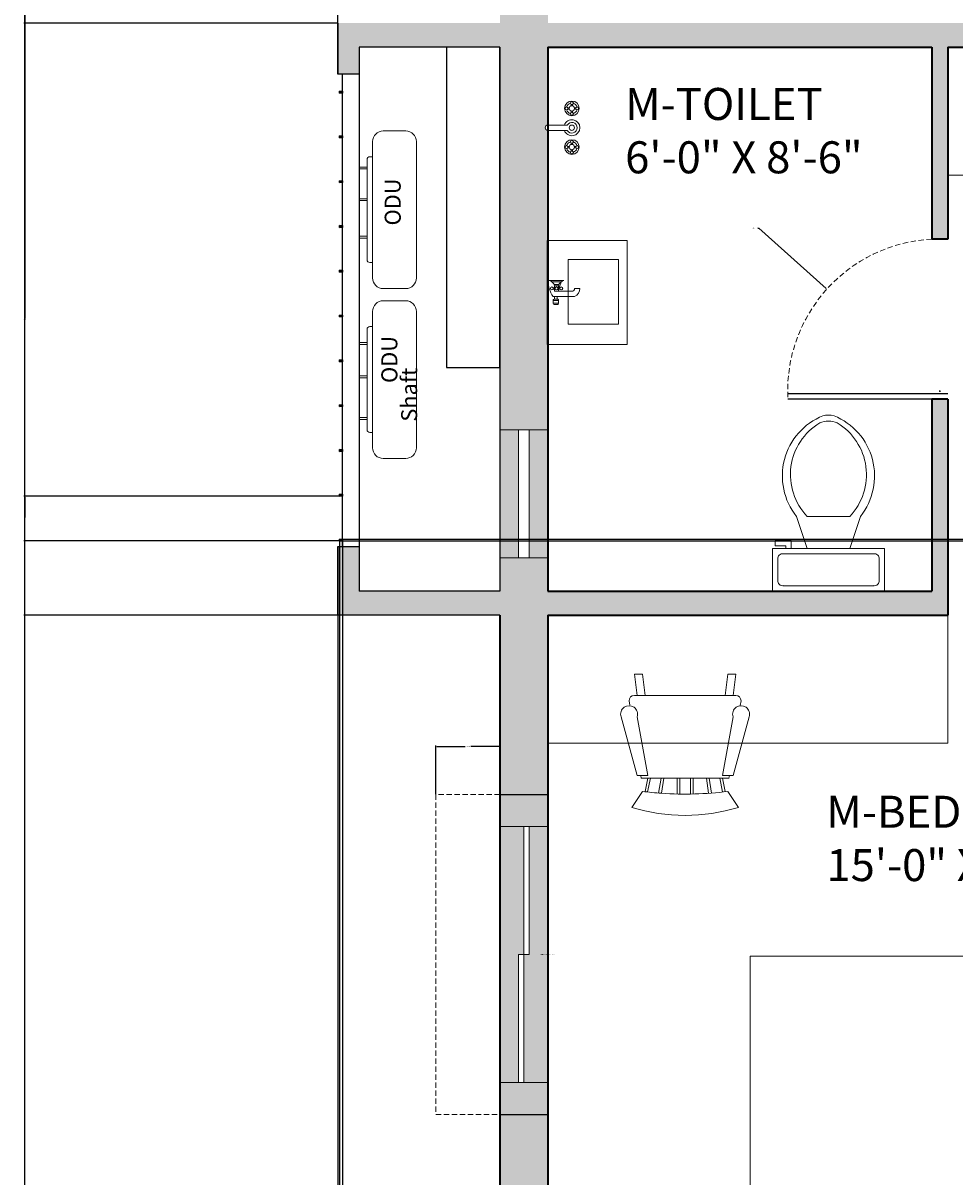
# Model space of a CAD drawing. Units: inches. Extents: x 1693 to 2974, y 2201 to 2965.
# Tile 2 of 24: x 1693 to 1868, y 2337 to 2554. Entities that reach past the tile are written whole.
import ezdxf

# ---------------------------------------------------------------- set-up
doc = ezdxf.new("R2010")
doc.units = ezdxf.units.IN
doc.header["$LTSCALE"] = 2
doc.header["$MEASUREMENT"] = 0
doc.linetypes.add('HIDDEN', pattern=[0.375, 0.25, -0.125])
for name, color, linetype, lineweight in [('A-ANNO-DIMS', 2, 'Continuous', 18), ('A-ANNO-TEXT', 7, 'Continuous', 13), ('A-AREA-IDEN', 7, 'Continuous', 18), ('A-DOOR', 3, 'Continuous', 25), ('A-DOOR-SWNG', 3, 'HIDDEN', 13), ('A-FLOR-CASE', 32, 'Continuous', 18), ('A-FLOR-FIXT', 9, 'Continuous', 18), ('A-FLOR-SHFT', 7, 'Continuous', 25), ('A-FURN', 8, 'Continuous', 18), ('A-GLAZ', 4, 'Continuous', 18), ('A-GLAZ-OVHD', 8, 'HIDDEN', 13), ('A-WALL', 7, 'Continuous', 35), ('M-HVAC-EQPM', 151, 'Continuous', 18)]:
    doc.layers.add(name, color=color, linetype=linetype, lineweight=lineweight)
doc.layers.add('A-GLAZ-PATT', color=141, linetype='Continuous', lineweight=13, true_color=0xadddf7)
doc.layers.add('A-WALL-PATT', color=251, linetype='Continuous', lineweight=13, true_color=0x636466)
doc.styles.get("Standard").update_dxf_attribs({"font": 'arial.ttf'})
doc.dimstyles.get("Standard").update_dxf_attribs({"dimtxt": 0.18, "dimasz": 0.18, "dimexe": 0.18, "dimexo": 0.0625, "dimgap": 0.09, "dimtad": 0, "dimtih": 1, "dimtoh": 1, "dimdec": 1, "dimzin": 0, "dimdsep": 46, "dimlunit": 3, "dimtxsty": 'Standard', "dimcen": 0.09, "dimadec": 0, "dimazin": 0, "dimtfac": 1, "dimtdec": 1, "dimtofl": 0, "dimtmove": 0, "dimatfit": 3, "dimfxl": 1, "dimtolj": 1, "dimtzin": 0, "dimarcsym": 0})

# ---------------------------------------------------------------- blocks, each defined once
blk = doc.blocks.new('Bed - Queen')
for p, q in [((0, -80.00003), (0, 0)), ((0, 0), (59.99999, 0)), ((59.99999, 0), (59.99999, -80.00003)), ((7.99999, -1.2), (28.79998, -1.2)), ((7.99999, -14.4), (7.99999, -1.2)), ((28.79998, -1.2), (28.79998, -14.4)), ((31.19999, -1.2), (51.99999, -1.2)), ((31.19999, -14.4), (31.19999, -1.2)), ((51.99999, -1.2), (51.99999, -16.4)), ((0, -14.4), (44.8, -14.4)), ((59.99999, -29.6), (44.8, -14.4)), ((44.8, -14.4), (44.8, -29.6)), ((44.8, -16.8), (0, -16.8)), ((51.99999, -16.4), (46.79936, -16.4)), ((44.8, -29.6), (59.99999, -29.6)), ((59.99999, -80.00003), (0, -80.00003))]:
    blk.add_line(p, q)
blk = doc.blocks.new('Toilet - top')
for p, q in [((9.5, -6), (9.5, -2)), ((-10, -8.5), (-8, -8.5)), ((-10, -9.5), (-10, -8.5)), ((-8, -8.5), (-8, -8)), ((-7, -8), (-7, -9.5)), ((-4, -8), (-6, -14)), ((4, -8), (6, -14)), ((-7, -9.5), (-10, -9.5)), ((4, -14), (-4, -14))]:
    blk.add_line(p, q)
blk.add_lwpolyline([(10.5, -8), (10.5, 0), (-10.5, 0), (-10.5, -8)], close=True)
for points in [[(-9.5, -2), (-9.5, -6)], [(8.5, -1), (-8.5, -1)], [(-8.5, -7), (8.5, -7)]]:
    blk.add_lwpolyline(points)
for centre, radius, start, end in [((-8.62, -1.88), 0.884, 81.8699, 188.1301), ((8.62, -1.88), 0.884, 351.8699, 98.1301), ((-8.62, -6.12), 0.884, 171.8699, 278.1301), ((8.62, -6.12), 0.884, 261.8699, 8.1301), ((3.52, -21.58), 12.17, 141.4691, 247.9714), ((4.2, -21.82), 11.33, 136.3677, 238.9468), ((-3.52, -21.58), 12.17, 292.0284, 38.5307), ((-4.2, -21.82), 11.33, 301.053, 43.6321), ((0, -27.88), 4, 245.7318, 294.2682), ((0, -29), 4, 254.8605, 285.1395)]:
    blk.add_arc(centre, radius, start, end)
blk = doc.blocks.new('Faucet - Bathroom side')
for p, q in [((-0.625, 4.25), (0.375, 4.25)), ((0.375, 3.75), (-0.625, 3.75)), ((-0.625, 3), (3.375, 3)), ((-0.375, 3), (-0.375, 3.5)), ((0.125, 3.5), (0.125, 3)), ((-1.625, 0), (-1.375, 0)), ((-1.375, 0), (1.375, 0)), ((-0.88366, 0.25), (0.88424, 0.25)), ((-0.375, 1.625), (-0.625, 1.625)), ((-0.375, 1.375), (-0.625, 1.375)), ((0.48078, 0.75), (-0.47286, 0.75)), ((2.875, 2), (0.375, 2)), ((0.375, 1.625), (0.625, 1.625)), ((0.375, 1.375), (0.625, 1.375)), ((4.375, 1.5), (3.375, 1.5))]:
    blk.add_line(p, q)
for points in [[(-0.375, 4.5), (0.125, 4.5)], [(-0.625, 3.75), (-0.625, 4.25)], [(0.125, 3.5), (-0.375, 3.5)], [(0.375, 4.25), (0.375, 3.75)]]:
    blk.add_lwpolyline(points)
blk.add_lwpolyline([(-0.375, 1), (-0.375, 2), (0.375, 2), (0.375, 1)], close=True)
for centre in [(-0.875, 1.5), (0, 1.5), (0.875, 1.5)]:
    blk.add_circle(centre, 0.27951)
for centre, radius, start, end in [((-0.38253, 4.2575), 0.24259, 88.22243, 181.7776), ((0.13252, 4.2575), 0.24259, 358.2224, 91.77757), ((3.45929, -0.0281), 5.08436, 143.4467, 179.6834), ((-0.38253, 3.7424), 0.24259, 178.2224, 271.7776), ((0.13252, 3.7424), 0.24259, 268.2224, 1.777565), ((2.70708, 1.4714), 1.66816, 0.9827695, 66.39737), ((-1.75, 1.375), 1.42522, 285.2551, 344.7449), ((1.75, 1.375), 1.42522, 195.2551, 254.7449), ((-2.49562, -0.286), 3.38273, 9.709485, 29.48735), ((2.96867, 1.5936), 0.41699, 347.0192, 102.9808)]:
    blk.add_arc(centre, radius, start, end)
blk = doc.blocks.new('Faucet - Bathroom top')
for p, q in [((-4.107, 0.125), (-4.375, 0.125)), ((-3.75, 0.4788), (-3.75, 0.75)), ((-3.5, 0.482), (-3.5, 0.75)), ((-3.1461, 0.125), (-2.875, 0.125)), ((3.143, 0.125), (2.875, 0.125)), ((3.5, 0.4788), (3.5, 0.75)), ((3.75, 0.482), (3.75, 0.75)), ((4.1039, 0.125), (4.375, 0.125)), ((-4.1039, -0.125), (-4.375, -0.125)), ((-3.75, -0.4821), (-3.75, -0.75)), ((-3.5, -0.4789), (-3.5, -0.75)), ((-3.143, -0.125), (-2.875, -0.125)), ((-0.5, -0.8639), (-0.5, -4.5)), ((0.5, -4.5), (0.5, -0.8631)), ((3.1461, -0.125), (2.875, -0.125)), ((3.5, -0.4821), (3.5, -0.75)), ((3.75, -0.4789), (3.75, -0.75)), ((4.107, -0.125), (4.375, -0.125))]:
    blk.add_line(p, q)
for centre, radius in [((-3.625, 0), 1.375), ((-4.625, 0), 0.2795), ((-3.625, 0), 0.5), ((-3.625, 1), 0.2795), ((-2.625, 0), 0.2795), ((0, 0), 0.5), ((3.625, 0), 1.375), ((2.625, 0), 0.2795), ((3.625, 0), 0.5), ((3.625, 1), 0.2795), ((4.625, 0), 0.2795), ((-3.625, -1), 0.2795), ((3.625, -1), 0.2795)]:
    blk.add_circle(centre, radius)
for centre, radius, start, end in [((-3.625, 0), 1, 105.2407, 164.2093), ((-3.625, 0), 1, 16.44125, 74.07887), ((0, 0), 1.5, 289.6514, 250.3603), ((0, 0), 1, 300.3431, 239.7554), ((3.625, 0), 1, 106.12, 164.0884), ((3.625, 0), 1, 16.23422, 73.90469), ((-3.625, 0), 1, 196.2342, 253.9047), ((-3.625, 0), 1, 286.12, 344.0884), ((3.625, 0), 1, 196.4413, 254.0789), ((3.625, 0), 1, 285.2407, 344.2093), ((0, -4.5), 0.5, 180, 0)]:
    blk.add_arc(centre, radius, start, end)
blk = doc.blocks.new('Chair - Rocking')
for p, q in [((-8, -4.5), (-10, -1.5)), ((8, -4.5), (10, -1.5)), ((-4.5, -7), (-4.96674, -4.19951)), ((-4, -7), (-4.40532, -4.16272)), ((-1.5, -4.05012), (-1.5, -7)), ((-1, -7), (-1, -4.05012)), ((1, -7), (1, -4.04655)), ((1.5, -4.05012), (1.5, -7)), ((4, -7), (4.40187, -4.18694)), ((4.5, -7), (4.96761, -4.19437)), ((-7.5, -4.5), (-7, -7)), ((-6.5, -7), (-7.02225, -4.43)), ((6.5, -7), (7, -4.4057)), ((7.5, -4.5), (7, -7)), ((-9, -7.5), (-12, -18.49999)), ((-7, -7.5), (-9, -7.5)), ((-9, -18.49999), (-7, -7.5)), ((-8.23428, -6.99939), (-8.3093, -7.47958)), ((-8.23041, -7), (8.23915, -7)), ((7, -7.5), (9, -7.5)), ((9, -18.49999), (7, -7.5)), ((8.31071, -7.48854), (8.23449, -7.00073)), ((9, -7.5), (12, -18.49999)), ((-10.36644, -20.64523), (-10.5, -21.49999)), ((10.5, -21.49999), (10.3575, -20.58798)), ((-9, -22.49999), (-9.5, -26.49999)), ((0, -22.49999), (-9.5, -22.49999)), ((-8, -26.49999), (-7.5, -22.49999)), ((0, -22.49999), (9.5, -22.49999)), ((8, -26.49999), (7.5, -22.49999)), ((9, -22.49999), (9.5, -26.49999)), ((-9.5, -26.49999), (-8, -26.49999)), ((9.5, -26.49999), (8, -26.49999))]:
    blk.add_line(p, q)
for centre, radius, start, end in [((0, -34.08333), 34.08333, 72.93847, 107.0615), ((0, -68.25004), 64.25, 93.92211, 97.15267), ((0, -68.25004), 64.25, 82.84733, 93.92211), ((-10.5, -18.99999), 1.58114, 161.5651, 18.43495), ((10.5, -18.99999), 1.58114, 161.5651, 18.43495), ((-9.5, -21.49999), 1, 180, 270), ((9.5, -21.49999), 1, 270, 0)]:
    blk.add_arc(centre, radius, start, end)
blk = doc.blocks.new('CONDENSER-WITH-BRACKETS')
at = {"ltscale": 2}
for points in [[(2, 10.74), (27.57, 10.74, -0.414214), (29.57, 8.74), (29.57, 4.53, -0.414214), (27.57, 2.53), (2, 2.53, -0.414214), (0, 4.53), (0, 8.74, -0.414214)], [(4.85, 2.53), (24.67, 2.53), (24.67, 2, -0.414214), (24.17, 1.5), (5.35, 1.5, -0.414214), (4.85, 2)]]:
    blk.add_lwpolyline(points, format="xyb", close=True, dxfattribs=at)
for points in [[(7.84, 1.5), (8.19, 1.5), (8.19, 0), (7.84, 0)], [(14.1, 1.5), (14.45, 1.5), (14.45, 0), (14.1, 0)], [(21.89, 1.5), (22.24, 1.5), (22.24, 0), (21.89, 0)]]:
    blk.add_lwpolyline(points, close=True, dxfattribs=at)
blk = doc.blocks.new('SHAFT-GUARD-POST-B')
at = {"ltscale": 2}
for p, q in [((0.55, 0), (0, 0.36)), ((0, 0), (0.55, 0.36))]:
    blk.add_line(p, q, dxfattribs=at)
blk.add_lwpolyline([(0.55, 0), (0, 0), (0, 0.36), (0.55, 0.36)], close=True, dxfattribs=at)
blk = doc.blocks.new('WINDOW-HOOD-60IN')
at = {"ltscale": 2}
for p, q in [((6, 12), (0, 12)), ((0, 12), (0, 0)), ((60, 12), (6, 12)), ((60, 0), (60, 12)), ((54, 0), (60, 0))]:
    blk.add_line(p, q, dxfattribs=at)
blk = doc.blocks.new('*D49')
at = {"layer": 'A-ANNO-DIMS', "color": 0, "lineweight": -2, "ltscale": 2, "transparency": 16777216}
for p, q in [((1782.8, 2409.19), (1791.92, 2409.19)), ((1791.74, 2409.01), (1791.74, 2379.38)), ((1791.74, 2349.37), (1791.74, 2379.01)), ((1782.8, 2349.19), (1791.92, 2349.19))]:
    blk.add_line(p, q, dxfattribs=at)
at = {"layer": 'A-ANNO-DIMS', "color": 0, "ltscale": 2, "transparency": 16777216}
for points in [[(1791.71, 2409.01), (1791.77, 2409.01), (1791.74, 2409.19)], [(1791.71, 2349.37), (1791.77, 2349.37), (1791.74, 2349.19)]]:
    blk.add_solid(points, dxfattribs=at)
at = {"layer": 'Defpoints', "color": 0, "ltscale": 2, "transparency": 16777216}
for p in [(1782.74, 2409.19), (1791.74, 2409.19), (1782.74, 2349.19)]:
    blk.add_point(p, dxfattribs=at)
at = {"layer": 'A-ANNO-DIMS', "color": 0, "ltscale": 2, "transparency": 16777216, "insert": (1791.74, 2379.19), "char_height": 0.18, "attachment_point": 5}
blk.add_mtext('\\A1;WINDOW HOOD A 60 TYP.', dxfattribs=at)
blk = doc.blocks.new('*D50')
at = {"layer": 'A-ANNO-DIMS', "color": 0, "lineweight": -2, "ltscale": 2, "transparency": 16777216}
for p, q in [((1770.74, 2409.25), (1770.74, 2418.37)), ((1770.92, 2418.19), (1776.22, 2418.19)), ((1782.56, 2418.19), (1777.26, 2418.19)), ((1782.74, 2409.25), (1782.74, 2418.37))]:
    blk.add_line(p, q, dxfattribs=at)
at = {"layer": 'A-ANNO-DIMS', "color": 0, "ltscale": 2, "transparency": 16777216}
for points in [[(1770.92, 2418.22), (1770.92, 2418.16), (1770.74, 2418.19)], [(1782.56, 2418.22), (1782.56, 2418.16), (1782.74, 2418.19)]]:
    blk.add_solid(points, dxfattribs=at)
at = {"layer": 'Defpoints', "color": 0, "ltscale": 2, "transparency": 16777216}
for p in [(1770.74, 2418.19), (1770.74, 2409.19), (1782.74, 2409.19)]:
    blk.add_point(p, dxfattribs=at)
at = {"layer": 'A-ANNO-DIMS', "color": 0, "ltscale": 2, "transparency": 16777216, "insert": (1776.74, 2418.19), "char_height": 0.18, "attachment_point": 5}
blk.add_mtext('\\A1;12 TYP.', dxfattribs=at)
blk = doc.blocks.new('*D81')
at = {"layer": 'A-ANNO-DIMS', "color": 0, "lineweight": -2, "ltscale": 2, "transparency": 16777216}
for p, q in [((1752.34, 2553.91), (1752.34, 2964.96)), ((1752.52, 2964.78), (2332.94, 2964.78)), ((2914.06, 2964.78), (2333.64, 2964.78)), ((2914.24, 2754.97), (2914.24, 2964.96))]:
    blk.add_line(p, q, dxfattribs=at)
at = {"layer": 'A-ANNO-DIMS', "color": 0, "ltscale": 2, "transparency": 16777216}
for points in [[(1752.52, 2964.81), (1752.52, 2964.75), (1752.34, 2964.78)], [(2914.06, 2964.81), (2914.06, 2964.75), (2914.24, 2964.78)]]:
    blk.add_solid(points, dxfattribs=at)
at = {"layer": 'Defpoints', "color": 0, "ltscale": 2, "transparency": 16777216}
for p in [(2914.24, 2964.78), (2914.24, 2754.9), (1752.34, 2553.84)]:
    blk.add_point(p, dxfattribs=at)
at = {"layer": 'A-ANNO-DIMS', "color": 0, "ltscale": 2, "transparency": 16777216, "insert": (2333.29, 2964.78), "char_height": 0.18, "attachment_point": 5}
blk.add_mtext('\\A1;1162', dxfattribs=at)
blk = doc.blocks.new('*D82')
at = {"layer": 'A-ANNO-DIMS', "color": 0, "lineweight": -2, "ltscale": 2, "transparency": 16777216}
for p, q in [((2615.67, 2906.08), (1693.46, 2906.08)), ((1693.64, 2905.9), (1693.64, 2582.94)), ((1693.64, 2259.62), (1693.64, 2582.58)), ((2096.17, 2259.44), (1693.46, 2259.44))]:
    blk.add_line(p, q, dxfattribs=at)
at = {"layer": 'A-ANNO-DIMS', "color": 0, "ltscale": 2, "transparency": 16777216}
for points in [[(1693.61, 2905.9), (1693.67, 2905.9), (1693.64, 2906.08)], [(1693.61, 2259.62), (1693.67, 2259.62), (1693.64, 2259.44)]]:
    blk.add_solid(points, dxfattribs=at)
at = {"layer": 'Defpoints', "color": 0, "ltscale": 2, "transparency": 16777216}
for p in [(1693.64, 2906.08), (2615.74, 2906.08), (2096.24, 2259.44)]:
    blk.add_point(p, dxfattribs=at)
at = {"layer": 'A-ANNO-DIMS', "color": 0, "ltscale": 2, "transparency": 16777216, "insert": (1693.64, 2582.76), "char_height": 0.18, "attachment_point": 5}
blk.add_mtext('\\A1;646.6', dxfattribs=at)
blk = doc.blocks.new('*D86')
at = {"layer": 'A-ANNO-DIMS', "color": 0, "lineweight": -2, "ltscale": 2, "transparency": 16777216}
for p, q in [((1782.67, 2706.84), (1693.46, 2706.84)), ((1693.64, 2706.66), (1693.64, 2498.53)), ((1693.64, 2290.02), (1693.64, 2498.16)), ((1782.67, 2289.84), (1693.46, 2289.84))]:
    blk.add_line(p, q, dxfattribs=at)
at = {"layer": 'A-ANNO-DIMS', "color": 0, "ltscale": 2, "transparency": 16777216}
for points in [[(1693.61, 2706.66), (1693.67, 2706.66), (1693.64, 2706.84)], [(1693.61, 2290.02), (1693.67, 2290.02), (1693.64, 2289.84)]]:
    blk.add_solid(points, dxfattribs=at)
at = {"layer": 'Defpoints', "color": 0, "ltscale": 2, "transparency": 16777216}
for p in [(1693.64, 2706.84), (1782.74, 2706.84), (1782.74, 2289.84)]:
    blk.add_point(p, dxfattribs=at)
at = {"layer": 'A-ANNO-DIMS', "color": 0, "ltscale": 2, "transparency": 16777216, "insert": (1693.64, 2498.34), "char_height": 0.18, "attachment_point": 5}
blk.add_mtext('\\A1;417', dxfattribs=at)
blk = doc.blocks.new('*D92')
at = {"layer": 'A-ANNO-DIMS', "color": 0, "lineweight": -2, "ltscale": 2, "transparency": 16777216}
for p, q in [((1752.34, 2442.78), (1752.34, 2200.56)), ((1782.74, 2442.78), (1782.74, 2200.56)), ((1752.52, 2200.74), (1767.21, 2200.74)), ((1782.56, 2200.74), (1767.86, 2200.74))]:
    blk.add_line(p, q, dxfattribs=at)
at = {"layer": 'A-ANNO-DIMS', "color": 0, "ltscale": 2, "transparency": 16777216}
for points in [[(1752.52, 2200.77), (1752.52, 2200.71), (1752.34, 2200.74)], [(1782.56, 2200.77), (1782.56, 2200.71), (1782.74, 2200.74)]]:
    blk.add_solid(points, dxfattribs=at)
at = {"layer": 'Defpoints', "color": 0, "ltscale": 2, "transparency": 16777216}
for p in [(1752.34, 2442.84), (1782.74, 2442.84), (1782.74, 2200.74)]:
    blk.add_point(p, dxfattribs=at)
at = {"layer": 'A-ANNO-DIMS', "color": 0, "ltscale": 2, "transparency": 16777216, "insert": (1767.54, 2200.74), "char_height": 0.18, "attachment_point": 5}
blk.add_mtext('\\A1;30.4', dxfattribs=at)
blk = doc.blocks.new('*D93')
at = {"layer": 'A-ANNO-DIMS', "color": 0, "lineweight": -2, "ltscale": 2, "transparency": 16777216}
for p, q in [((1752.27, 2553.84), (1693.46, 2553.84)), ((1693.64, 2553.66), (1693.64, 2498.53)), ((1693.64, 2443.02), (1693.64, 2498.16)), ((1752.27, 2442.84), (1693.46, 2442.84))]:
    blk.add_line(p, q, dxfattribs=at)
at = {"layer": 'A-ANNO-DIMS', "color": 0, "ltscale": 2, "transparency": 16777216}
for points in [[(1693.61, 2553.66), (1693.67, 2553.66), (1693.64, 2553.84)], [(1693.61, 2443.02), (1693.67, 2443.02), (1693.64, 2442.84)]]:
    blk.add_solid(points, dxfattribs=at)
at = {"layer": 'Defpoints', "color": 0, "ltscale": 2, "transparency": 16777216}
for p in [(1693.64, 2553.84), (1752.34, 2553.84), (1752.34, 2442.84)]:
    blk.add_point(p, dxfattribs=at)
at = {"layer": 'A-ANNO-DIMS', "color": 0, "ltscale": 2, "transparency": 16777216, "insert": (1693.64, 2498.34), "char_height": 0.18, "attachment_point": 5}
blk.add_mtext('\\A1;111', dxfattribs=at)
blk = doc.blocks.new('*D106')
at = {"layer": 'A-ANNO-DIMS', "color": 0, "lineweight": -2, "ltscale": 2, "transparency": 16777216}
for p, q in [((1752.61, 2465.13), (1693.46, 2465.13)), ((1693.64, 2464.95), (1693.64, 2461.11)), ((1693.64, 2456.91), (1693.64, 2460.75)), ((1752.61, 2456.73), (1693.46, 2456.73))]:
    blk.add_line(p, q, dxfattribs=at)
at = {"layer": 'A-ANNO-DIMS', "color": 0, "ltscale": 2, "transparency": 16777216}
for points in [[(1693.61, 2464.95), (1693.67, 2464.95), (1693.64, 2465.13)], [(1693.61, 2456.91), (1693.67, 2456.91), (1693.64, 2456.73)]]:
    blk.add_solid(points, dxfattribs=at)
at = {"layer": 'Defpoints', "color": 0, "ltscale": 2, "transparency": 16777216}
for p in [(1693.64, 2465.13), (1752.68, 2465.13), (1752.68, 2456.73)]:
    blk.add_point(p, dxfattribs=at)
at = {"layer": 'A-ANNO-DIMS', "color": 0, "ltscale": 2, "transparency": 16777216, "insert": (1693.64, 2460.93), "char_height": 0.18, "attachment_point": 5}
blk.add_mtext('\\A1;8.4', dxfattribs=at)
blk = doc.blocks.new('*D107')
at = {"layer": 'A-ANNO-DIMS', "color": 0, "lineweight": -2, "ltscale": 2, "transparency": 16777216}
for p, q in [((1752.68, 2456.67), (1752.68, 2200.56)), ((1753.22, 2456.67), (1753.22, 2200.56)), ((1752.86, 2200.74), (1753.04, 2200.74)), ((1753.22, 2200.74), (1753.4, 2200.74))]:
    blk.add_line(p, q, dxfattribs=at)
at = {"layer": 'A-ANNO-DIMS', "color": 0, "ltscale": 2, "transparency": 16777216}
for points in [[(1752.86, 2200.77), (1752.86, 2200.71), (1752.68, 2200.74)], [(1753.04, 2200.77), (1753.04, 2200.71), (1753.22, 2200.74)]]:
    blk.add_solid(points, dxfattribs=at)
at = {"layer": 'Defpoints', "color": 0, "ltscale": 2, "transparency": 16777216}
for p in [(1752.68, 2456.73), (1753.22, 2456.73), (1753.22, 2200.74)]:
    blk.add_point(p, dxfattribs=at)
at = {"layer": 'A-ANNO-DIMS', "color": 0, "ltscale": 2, "transparency": 16777216, "insert": (1753.8, 2200.74), "char_height": 0.18, "attachment_point": 5}
blk.add_mtext('\\A1;0.547', dxfattribs=at)
blk = doc.blocks.new('*D108')
at = {"layer": 'A-ANNO-DIMS', "color": 0, "lineweight": -2, "ltscale": 2, "transparency": 16777216}
for p, q in [((1752.74, 2457.09), (2973.12, 2457.09)), ((1752.74, 2456.73), (2973.12, 2456.73)), ((2972.94, 2457.27), (2972.94, 2457.45)), ((2972.94, 2457.45), (2973.12, 2457.45)), ((2972.94, 2456.55), (2972.94, 2456.37))]:
    blk.add_line(p, q, dxfattribs=at)
at = {"layer": 'A-ANNO-DIMS', "color": 0, "ltscale": 2, "transparency": 16777216}
for points in [[(2972.91, 2457.27), (2972.97, 2457.27), (2972.94, 2457.09)], [(2972.91, 2456.55), (2972.97, 2456.55), (2972.94, 2456.73)]]:
    blk.add_solid(points, dxfattribs=at)
at = {"layer": 'Defpoints', "color": 0, "ltscale": 2, "transparency": 16777216}
for p in [(1752.68, 2457.09), (1752.68, 2456.73), (2972.94, 2457.09)]:
    blk.add_point(p, dxfattribs=at)
at = {"layer": 'A-ANNO-DIMS', "color": 0, "ltscale": 2, "transparency": 16777216, "insert": (2973.44, 2457.45), "char_height": 0.18, "attachment_point": 5}
blk.add_mtext('\\A1;0.36', dxfattribs=at)
blk = doc.blocks.new('*D124')
at = {"layer": 'A-ANNO-DIMS', "color": 0, "lineweight": -2, "ltscale": 2, "transparency": 16777216}
for p, q in [((1831.11, 2515.39), (1831.29, 2515.39)), ((1831.29, 2515.39), (1843.89, 2504.06)), ((1865.15, 2484.84), (1865.33, 2484.84)), ((1865.24, 2484.75), (1865.24, 2484.93))]:
    blk.add_line(p, q, dxfattribs=at)
at = {"layer": 'A-ANNO-DIMS', "color": 0, "ltscale": 2, "transparency": 16777216}
blk.add_solid([(1843.91, 2504.08), (1843.87, 2504.03), (1844.03, 2503.93)], dxfattribs=at)
at = {"layer": 'Defpoints', "color": 0, "ltscale": 2, "transparency": 16777216}
for p in [(1844.03, 2503.93), (1865.24, 2484.84)]:
    blk.add_point(p, dxfattribs=at)
at = {"layer": 'A-ANNO-DIMS', "color": 0, "ltscale": 2, "transparency": 16777216, "insert": (1830.56, 2515.39), "char_height": 0.18, "attachment_point": 5}
blk.add_mtext('\\A1;R28.547', dxfattribs=at)

msp = doc.modelspace()

# ---------------------------------------------------------------- hatches: boundary and pattern name
at = {"layer": 'A-GLAZ-PATT', "ltscale": 2}
h = msp.add_hatch(color=256, dxfattribs=at)
h.dxf.hatch_style = 1
h.paths.add_polyline_path([(2656.9702, 2338.2547), (2632.9702, 2338.2547), (2632.9702, 2339.2547), (2608.9702, 2339.2547), (2608.9702, 2334.7547), (2656.9702, 2334.7547)])
h.paths.add_polyline_path([(2656.9702, 2343.7547), (2608.9702, 2343.7547), (2608.9702, 2340.2547), (2632.9702, 2340.2547), (2632.9702, 2339.2547), (2656.9702, 2339.2547)])
h.paths.add_polyline_path([(2775.7544, 2338.2547), (2751.7544, 2338.2547), (2751.7544, 2334.7547), (2775.7544, 2334.7547)])
h.paths.add_polyline_path([(2775.7544, 2343.7547), (2751.7544, 2343.7547), (2751.7544, 2340.2547), (2775.7544, 2340.2547)])
h.paths.add_polyline_path([(2897.7363, 2568.7999), (2893.2363, 2568.7999), (2893.2363, 2520.7999), (2896.7363, 2520.7999), (2896.7363, 2544.7999), (2897.7363, 2544.7999)])
h.paths.add_polyline_path([(2902.2363, 2568.7999), (2898.7363, 2568.7999), (2898.7363, 2544.7999), (2897.7363, 2544.7999), (2897.7363, 2520.7999), (2902.2363, 2520.7999)])
h.paths.add_polyline_path([(2902.2363, 2637.7547), (2898.7363, 2637.7547), (2898.7363, 2613.7547), (2902.2363, 2613.7547)])
h.paths.add_polyline_path([(2896.7363, 2637.7547), (2893.2363, 2637.7547), (2893.2363, 2613.7547), (2896.7363, 2613.7547)])
h.paths.add_polyline_path([(2902.2363, 2748.903), (2899.0477, 2748.903), (2899.0477, 2724.903), (2898.0477, 2724.903), (2898.0477, 2700.903), (2902.2363, 2700.903)])
h.paths.add_polyline_path([(2898.0477, 2748.903), (2893.2363, 2748.903), (2893.2363, 2700.903), (2897.0477, 2700.903), (2897.0477, 2724.903), (2898.0477, 2724.903)])
h.paths.add_polyline_path([(2851.2363, 2846.2547), (2803.2363, 2846.2547), (2803.2363, 2842.7547), (2827.2363, 2842.7547), (2827.2363, 2841.7547), (2851.2363, 2841.7547)])
h.paths.add_polyline_path([(2851.2363, 2840.7547), (2827.2363, 2840.7547), (2827.2363, 2841.7547), (2803.2363, 2841.7547), (2803.2363, 2837.2547), (2851.2363, 2837.2547)])
h.paths.add_polyline_path([(2578.2363, 2846.2547), (2530.2363, 2846.2547), (2530.2363, 2842.7547), (2554.2363, 2842.7547), (2554.2363, 2841.7547), (2578.2363, 2841.7547)])
h.paths.add_polyline_path([(2578.2363, 2840.7547), (2554.2363, 2840.7547), (2554.2363, 2841.7547), (2530.2363, 2841.7547), (2530.2363, 2837.2547), (2578.2363, 2837.2547)])
h.paths.add_polyline_path([(2732.7363, 2812.7547), (2705.1363, 2812.7547), (2705.1363, 2811.7547), (2676.3363, 2811.7547), (2676.3363, 2812.7547), (2648.7363, 2812.7547), (2648.7363, 2808.2547), (2732.7363, 2808.2547)])
h.paths.add_polyline_path([(2732.7363, 2817.2547), (2648.7363, 2817.2547), (2648.7363, 2813.7547), (2676.3363, 2813.7547), (2676.3363, 2812.7547), (2705.1363, 2812.7547), (2705.1363, 2813.7547), (2732.7363, 2813.7547)])
h.paths.add_polyline_path([(2488.2363, 2695.8203), (2484.7878, 2695.8203), (2484.7878, 2671.8203), (2488.2363, 2671.8203)])
h.paths.add_polyline_path([(2482.7878, 2695.8203), (2479.2363, 2695.8203), (2479.2363, 2671.8203), (2482.7878, 2671.8203)])
h.paths.add_polyline_path([(2488.2363, 2572.4371), (2484.7363, 2572.4371), (2484.7363, 2541.4371), (2483.7363, 2541.4371), (2483.7363, 2512.4371), (2488.2363, 2512.4371)])
h.paths.add_polyline_path([(2482.7363, 2541.4371), (2483.7363, 2541.4371), (2483.7363, 2572.4371), (2479.2363, 2572.4371), (2479.2363, 2512.4371), (2482.7363, 2512.4371)])
h.paths.add_polyline_path([(2248.9863, 2706.8449), (2190.9863, 2706.8449), (2190.9863, 2703.3449), (2219.9863, 2703.3449), (2219.9863, 2702.3449), (2248.9863, 2702.3449)])
h.paths.add_polyline_path([(2248.9863, 2701.3449), (2219.9863, 2701.3449), (2219.9863, 2702.3449), (2190.9863, 2702.3449), (2190.9863, 2697.8449), (2248.9863, 2697.8449)])
h.paths.add_polyline_path([(2151.9207, 2293.3449), (2127.9207, 2293.3449), (2127.9207, 2289.8449), (2151.9207, 2289.8449)])
h.paths.add_polyline_path([(2151.9207, 2298.8449), (2127.9207, 2298.8449), (2127.9207, 2295.3449), (2151.9207, 2295.3449)])
h.paths.add_polyline_path([(2084.023, 2293.3449), (2066.023, 2293.3449), (2066.023, 2294.3449), (2048.023, 2294.3449), (2048.023, 2289.8449), (2084.023, 2289.8449)])
h.paths.add_polyline_path([(2084.023, 2298.8449), (2048.023, 2298.8449), (2048.023, 2295.3449), (2066.023, 2295.3449), (2066.023, 2294.3449), (2084.023, 2294.3449)])
h.paths.add_polyline_path([(1966.0781, 2293.3449), (1948.0781, 2293.3449), (1948.0781, 2294.3449), (1930.0781, 2294.3449), (1930.0781, 2289.8449), (1966.0781, 2289.8449)])
h.paths.add_polyline_path([(1966.0781, 2298.8449), (1930.0781, 2298.8449), (1930.0781, 2295.3449), (1948.0781, 2295.3449), (1948.0781, 2294.3449), (1966.0781, 2294.3449)])
h.paths.add_polyline_path([(1787.2363, 2403.1922), (1782.7363, 2403.1922), (1782.7363, 2355.1922), (1786.2363, 2355.1922), (1786.2363, 2379.1922), (1787.2363, 2379.1922)])
h.paths.add_polyline_path([(1791.7363, 2403.1922), (1788.2363, 2403.1922), (1788.2363, 2379.1922), (1787.2363, 2379.1922), (1787.2363, 2355.1922), (1791.7363, 2355.1922)])
h.paths.add_polyline_path([(1786.2363, 2477.5455), (1782.7363, 2477.5455), (1782.7363, 2453.5455), (1786.2363, 2453.5455)])
h.paths.add_polyline_path([(1791.7363, 2477.5455), (1788.2363, 2477.5455), (1788.2363, 2453.5455), (1791.7363, 2453.5455)])
h.paths.add_polyline_path([(1786.2363, 2621.6433), (1782.7363, 2621.6433), (1782.7363, 2585.6433), (1786.2363, 2585.6433)])
h.paths.add_polyline_path([(1791.7363, 2621.6433), (1788.2363, 2621.6433), (1788.2363, 2585.6433), (1791.7363, 2585.6433)])
h.paths.add_polyline_path([(1908.1286, 2706.8449), (1860.1286, 2706.8449), (1860.1286, 2703.3449), (1884.1286, 2703.3449), (1884.1286, 2702.3449), (1908.1286, 2702.3449)])
h.paths.add_polyline_path([(1908.1286, 2701.3449), (1884.1286, 2701.3449), (1884.1286, 2702.3449), (1860.1286, 2702.3449), (1860.1286, 2697.8449), (1908.1286, 2697.8449)])
h.paths.add_polyline_path([(1973.9863, 2706.8449), (1949.9863, 2706.8449), (1949.9863, 2703.3449), (1973.9863, 2703.3449)])
h.paths.add_polyline_path([(1973.9863, 2701.3449), (1949.9863, 2701.3449), (1949.9863, 2697.8449), (1973.9863, 2697.8449)])
h.paths.add_polyline_path([(2112.7363, 2690.3449), (2028.7363, 2690.3449), (2028.7363, 2686.8449), (2056.3363, 2686.8449), (2056.3363, 2685.8449), (2085.1363, 2685.8449), (2085.1363, 2686.8449), (2112.7363, 2686.8449)])
h.paths.add_polyline_path([(2112.7363, 2685.8449), (2085.1363, 2685.8449), (2085.1363, 2684.8449), (2056.3363, 2684.8449), (2056.3363, 2685.8449), (2028.7363, 2685.8449), (2028.7363, 2681.3449), (2112.7363, 2681.3449)])
h.paths.add_polyline_path([(2422.7363, 2640.7547), (2350.7363, 2640.7547), (2350.7363, 2637.2547), (2386.7363, 2637.2547), (2386.7363, 2636.2547), (2422.7363, 2636.2547)])
h.paths.add_polyline_path([(2422.7363, 2635.2547), (2386.7363, 2635.2547), (2386.7363, 2636.2547), (2350.7363, 2636.2547), (2350.7363, 2631.7547), (2422.7363, 2631.7547)])
at = {"layer": 'A-WALL-PATT', "ltscale": 2}
h = msp.add_hatch(color=256, dxfattribs=at)
h.dxf.hatch_style = 1
h.paths.add_polyline_path([(1928.2363, 2733.2161), (1930.9384, 2733.2161), (1930.9384, 2737.2161), (1923.7363, 2737.2161), (1923.7363, 2706.8449), (1908.1286, 2706.8449), (1908.1286, 2697.8449), (1923.7363, 2697.8449), (1923.7363, 2692.8449), (1928.2363, 2692.8449), (1928.2363, 2697.8449), (1949.9863, 2697.8449), (1949.9863, 2706.8449), (1928.2363, 2706.8449)])
h.paths.add_polyline_path([(2004.7363, 2737.2161), (1995.7363, 2737.2161), (1995.7363, 2706.8449), (1985.6374, 2706.8449), (1973.9863, 2706.8449), (1973.9863, 2697.8449), (2000.2363, 2697.8449), (2000.2363, 2686.5348), (2000.3613, 2686.5348), (2000.3613, 2667.0432), (2000.2363, 2601.8449), (1928.2363, 2601.8449), (1928.2363, 2662.8449), (1923.7363, 2662.8449), (1923.7363, 2595.3449), (1928.2363, 2595.3449), (1928.2363, 2597.3449), (2004.7363, 2597.3449), (2004.7363, 2681.3449), (2012.7814, 2681.3449), (2028.7363, 2681.3449), (2028.7363, 2690.3449), (2004.7363, 2690.3449)])
h.paths.add_polyline_path([(2190.9863, 2706.8449), (2184.9863, 2706.8449), (2145.7363, 2706.8449), (2145.7363, 2765.3449), (2145.7363, 2774.5394), (2136.7363, 2774.5394), (2136.7363, 2756.3449), (2136.7363, 2690.3449), (2112.7363, 2690.3449), (2112.7363, 2681.3449), (2136.7363, 2681.3449), (2136.7363, 2597.3449), (2141.2363, 2597.3449), (2141.2363, 2697.8449), (2190.9863, 2697.8449)])
h.paths.add_polyline_path([(1860.1286, 2706.8449), (1782.7363, 2706.8449), (1782.7363, 2621.6433), (1791.7363, 2621.6433), (1791.7363, 2697.8449), (1860.1286, 2697.8449)])
h.paths.add_polyline_path([(1791.7363, 2585.6433), (1782.7363, 2585.6433), (1782.7363, 2562.8449), (1782.7363, 2553.8449), (1752.3363, 2553.8449), (1752.3363, 2544.2586), (1756.3363, 2544.2586), (1756.3363, 2549.3449), (1782.7363, 2549.3449), (1782.7363, 2489.2404), (1782.7363, 2477.5455), (1791.7363, 2477.5455), (1791.7363, 2493.5991), (1791.6113, 2493.5991), (1791.6113, 2513.0907), (1791.6824, 2533.7198, -0.94742783), (1791.7363, 2534.7168), (1791.7363, 2549.3449), (1863.7363, 2549.3449), (1863.7363, 2513.3449), (1866.7363, 2513.3449), (1866.7363, 2549.3449), (1924.7363, 2549.3449), (1924.7363, 2447.3449), (1924.7363, 2442.8449), (1933.7363, 2442.8449), (1933.7363, 2447.3449), (1928.2363, 2447.3449), (1928.2363, 2559.3449), (1923.7363, 2559.3449), (1923.7363, 2553.8449), (1791.7363, 2553.8449), (1791.7363, 2562.8449)])
h.paths.add_polyline_path([(1791.7363, 2442.8449), (1866.7363, 2442.8449), (1866.7363, 2447.3449), (1866.7363, 2483.3449), (1863.7363, 2483.3449), (1863.7363, 2447.3449), (1791.7363, 2447.3449), (1791.7363, 2453.5455), (1782.7363, 2453.5455), (1782.7363, 2447.3449), (1756.3363, 2447.3449), (1756.3363, 2455.7126), (1752.3363, 2455.7126), (1752.3363, 2442.8449), (1782.7363, 2442.8449), (1782.7363, 2403.1922), (1791.7363, 2403.1922)])
h.paths.add_polyline_path([(1930.0781, 2298.8449), (1791.7363, 2298.8449), (1791.7363, 2355.1922), (1782.7363, 2355.1922), (1782.7363, 2289.8449), (1930.0781, 2289.8449)])
h.paths.add_polyline_path([(2624.7363, 2883.2547), (2624.7363, 2902.6165), (2624.7363, 2906.0761), (2615.7363, 2906.0761), (2615.7363, 2892.2547), (2615.7363, 2846.2547), (2578.2363, 2846.2547), (2578.2363, 2837.2547), (2620.2363, 2837.2547), (2620.2363, 2743.2547), (2624.7363, 2743.2547), (2624.7363, 2808.2547), (2648.7363, 2808.2547), (2648.7363, 2817.2547), (2624.7363, 2817.2547)])
h.paths.add_polyline_path([(2530.2363, 2846.2547), (2479.2363, 2846.2547), (2479.2363, 2695.8203), (2488.2363, 2695.8203), (2488.2363, 2700.7547), (2567.2363, 2700.7547), (2567.2363, 2705.2547), (2488.2363, 2705.2547), (2488.2363, 2837.2547), (2530.2363, 2837.2547)])
h.paths.add_polyline_path([(2488.2363, 2487.7547), (2630.2363, 2487.7547, -0.00990191), (2630.2363, 2489.0322), (2630.2363, 2492.2547), (2488.2363, 2492.2547), (2488.2363, 2512.4371), (2479.2363, 2512.4371), (2479.2363, 2334.7547), (2608.9702, 2334.7547), (2608.9702, 2343.7547), (2488.2363, 2343.7547)])
h.paths.add_polyline_path([(2751.7544, 2343.7547), (2672.7363, 2343.7547), (2672.7363, 2409.7547), (2674.7363, 2409.7547), (2674.7363, 2413.7547), (2672.7363, 2413.7547), (2672.7363, 2487.7547), (2732.7363, 2487.7547), (2732.7363, 2413.7547), (2704.7363, 2413.7547), (2704.7363, 2409.7547), (2784.7363, 2409.7547), (2784.7363, 2343.7547), (2775.7544, 2343.7547), (2775.7544, 2334.7547), (2902.2363, 2334.7547), (2902.2363, 2520.7999), (2893.2363, 2520.7999), (2893.2363, 2413.7547), (2856.0145, 2413.7547), (2856.0145, 2409.7547), (2893.2363, 2409.7547), (2893.2363, 2343.7547), (2789.2363, 2343.7547), (2789.2363, 2409.7547), (2819.2363, 2409.7547), (2826.0145, 2409.7547), (2826.0145, 2413.7547), (2789.2363, 2413.7547), (2789.2363, 2492.2547), (2784.7363, 2492.2547), (2784.7363, 2413.7547), (2736.7363, 2413.7547), (2736.7363, 2492.2547), (2672.7363, 2492.2547), (2666.2363, 2492.2547), (2666.2363, 2487.7547), (2668.2363, 2487.7547), (2668.2363, 2343.7547), (2656.9702, 2343.7547), (2656.9702, 2334.7547), (2662.9702, 2334.7547), (2751.7544, 2334.7547)])
h.paths.add_polyline_path([(2902.2363, 2613.7547), (2893.2363, 2613.7547), (2893.2363, 2589.7547), (2785.2363, 2589.7547), (2785.2363, 2661.7547), (2790.2363, 2661.7547), (2790.2363, 2665.2547), (2761.2363, 2665.2547), (2761.2363, 2667.2547), (2756.7363, 2667.2547), (2756.7363, 2661.7547), (2781.2363, 2661.7547), (2781.2363, 2585.7547), (2893.2363, 2585.7547), (2893.2363, 2568.7999), (2902.2363, 2568.7999)])
h.paths.add_polyline_path([(2488.2363, 2671.8203), (2479.2363, 2671.8203), (2479.2363, 2645.2547), (2479.2363, 2623.4598), (2488.2363, 2623.4598), (2488.2363, 2636.2547), (2624.7363, 2636.2547), (2624.7363, 2640.7547), (2603.7363, 2640.7547), (2603.7363, 2700.7547), (2624.7363, 2700.7547), (2624.7363, 2707.2547), (2620.2363, 2707.2547), (2620.2363, 2705.2547), (2597.2363, 2705.2547), (2597.2363, 2700.7547), (2599.2363, 2700.7547), (2599.2363, 2640.7547), (2488.2363, 2640.7547)])
h.paths.add_polyline_path([(2761.2363, 2837.2547), (2803.2363, 2837.2547), (2803.2363, 2846.2547), (2797.2363, 2846.2547), (2765.7363, 2846.2547), (2756.7363, 2846.2547), (2756.7363, 2817.2547), (2732.7363, 2817.2547), (2732.7363, 2808.2547), (2756.7363, 2808.2547), (2756.7363, 2703.2547), (2761.2363, 2703.2547)])
h.paths.add_polyline_path([(2739.7489, 2433.1234), (2786.9181, 2433.1234), (2786.9181, 2455.5122), (2739.7489, 2455.5122)], flags=25)

# ---------------------------------------------------------------- linework, layer by layer
at = {"layer": 'A-DOOR', "ltscale": 2}
for p, q in [((1866.7363, 2484.3449), (1836.7363, 2484.3449)), ((1866.7363, 2483.3449), (1836.7363, 2483.3449))]:
    msp.add_line(p, q, dxfattribs=at)
at = {"layer": 'A-DOOR-SWNG', "ltscale": 2}
msp.add_arc((1865.2438, 2484.8381), 28.5466, 93.027167, 182.998408, dxfattribs=at)
at = {"layer": 'A-FLOR-CASE'}
for p, q in [((1866.7363, 2525.3449), (1900.7363, 2525.3449)), ((1791.7363, 2418.8449), (1866.7363, 2418.8449))]:
    msp.add_line(p, q, dxfattribs=at)
at = {"layer": 'A-FLOR-CASE', "ltscale": 2}
msp.add_line((1866.7363, 2442.8449), (1866.7363, 2418.8449), dxfattribs=at)
at = {"layer": 'A-FLOR-FIXT', "ltscale": 2}
for points in [[(1791.6113, 2513.0907), (1806.6251, 2513.0907), (1806.6251, 2493.5991), (1791.6113, 2493.5991)], [(1795.5241, 2509.537), (1804.9933, 2509.537), (1804.9933, 2497.3547), (1795.5241, 2497.3547)]]:
    msp.add_lwpolyline(points, close=True, dxfattribs=at)
at = {"layer": 'A-FLOR-SHFT', "ltscale": 2}
for p, q in [((1752.3363, 2553.8449), (1752.3363, 2544.2586)), ((1752.3363, 2544.2586), (1752.3363, 2553.8449)), ((1756.3363, 2549.3449), (1756.3363, 2544.2586)), ((1782.7363, 2549.3449), (1756.3363, 2549.3449)), ((1756.3363, 2544.2586), (1752.3363, 2544.2586)), ((1753.2225, 2455.7126), (1753.2225, 2544.2586)), ((1756.3363, 2544.2586), (1756.3363, 2455.7126)), ((1752.3363, 2442.8449), (1752.3363, 2455.7126)), ((1752.3363, 2455.7126), (1756.3363, 2455.7126)), ((1752.3363, 2455.7126), (1752.3363, 2442.8449)), ((1756.3363, 2455.7126), (1756.3363, 2447.3449)), ((1782.7363, 2447.3449), (1756.3363, 2447.3449)), ((1782.7363, 2442.8449), (1752.3363, 2442.8449))]:
    msp.add_line(p, q, dxfattribs=at)
at = {"layer": 'A-FLOR-SHFT'}
msp.add_line((1782.7363, 2549.3449), (1782.7363, 2447.3449), dxfattribs=at)
at = {"layer": 'A-FLOR-SHFT', "ltscale": 2}
msp.add_lwpolyline([(1782.7363, 2549.3449), (1772.7229, 2549.3449), (1772.7229, 2489.2404), (1782.7363, 2489.2404)], close=True, dxfattribs=at)
at = {"layer": 'A-GLAZ', "ltscale": 2}
for p, q in [((1782.7363, 2477.5455), (1791.7363, 2477.5455)), ((1786.2363, 2477.5455), (1786.2363, 2453.5455)), ((1788.2363, 2477.5455), (1788.2363, 2453.5455)), ((1782.7363, 2453.5455), (1791.7363, 2453.5455)), ((1791.7363, 2403.1922), (1782.7363, 2403.1922)), ((1787.2363, 2403.1922), (1787.2363, 2355.1922)), ((1788.2363, 2403.1922), (1788.2363, 2379.1922)), ((1788.2363, 2379.1922), (1786.2363, 2379.1922)), ((1786.2363, 2379.1922), (1786.2363, 2355.1922)), ((1791.7363, 2355.1922), (1782.7363, 2355.1922))]:
    msp.add_line(p, q, dxfattribs=at)
at = {"layer": 'A-WALL'}
for p, q in [((1791.7363, 2549.3449), (1863.7363, 2549.3449)), ((1791.7363, 2549.3449), (1791.7363, 2447.3449)), ((1863.7363, 2549.3449), (1863.7363, 2513.3449)), ((1866.7363, 2549.3449), (1866.7363, 2513.3449)), ((1866.7363, 2549.3449), (1924.7363, 2549.3449)), ((1866.7363, 2513.3449), (1863.7363, 2513.3449)), ((1866.7363, 2483.3449), (1863.7363, 2483.3449)), ((1863.7363, 2483.3449), (1863.7363, 2447.3449)), ((1866.7363, 2483.3449), (1866.7363, 2447.3449)), ((1791.7363, 2447.3449), (1863.7363, 2447.3449)), ((1866.7363, 2447.3449), (1866.7363, 2442.8449)), ((1782.7363, 2442.8449), (1782.7363, 2289.8449)), ((1791.7363, 2442.8449), (1866.7363, 2442.8449)), ((1791.7363, 2442.8449), (1791.7363, 2298.8449)), ((1791.7363, 2442.8449), (1866.7363, 2442.8449))]:
    msp.add_line(p, q, dxfattribs=at)
at = {"layer": 'M-HVAC-EQPM', "ltscale": 2}
for points in [[(1767.079, 2531.6223), (1767.079, 2506.0495, -0.41421356), (1765.079, 2504.0495), (1760.867, 2504.0495, -0.41421356), (1758.867, 2506.0495), (1758.867, 2531.6223, -0.41421356), (1760.867, 2533.6223), (1765.079, 2533.6223, -0.41421356)], [(1758.867, 2528.7748), (1758.867, 2508.9531), (1758.3319, 2508.9531, -0.41421356), (1757.8319, 2509.4531), (1757.8319, 2528.2748, -0.41421356), (1758.3319, 2528.7748)]]:
    msp.add_lwpolyline(points, format="xyb", close=True, dxfattribs=at)
for points in [[(1757.8319, 2526.8548), (1757.8319, 2526.5015), (1756.3363, 2526.5015), (1756.3363, 2526.8548)], [(1757.8319, 2520.9021), (1757.8319, 2520.5487), (1756.3363, 2520.5487), (1756.3363, 2520.9021)], [(1757.8319, 2513.8621), (1757.8319, 2513.5087), (1756.3363, 2513.5087), (1756.3363, 2513.8621)]]:
    msp.add_lwpolyline(points, close=True, dxfattribs=at)

# ---------------------------------------------------------------- block references
at = {"layer": 'A-FLOR-FIXT', "ltscale": 2, "rotation": 270}
msp.add_blockref('Faucet - Bathroom top', (1796.2363, 2534.2168), dxfattribs=at)
at = {"layer": 'A-FLOR-FIXT', "ltscale": 2, "xscale": -1, "rotation": 180}
for name, p in [('Faucet - Bathroom side', (1793.3613, 2505.5803)), ('Toilet - top', (1844.3509, 2447.3449))]:
    msp.add_blockref(name, p, dxfattribs=at)
at = {"layer": 'A-FLOR-SHFT'}
for p in [(1752.675, 2540.73), (1752.675, 2532.33), (1752.675, 2523.93), (1752.675, 2515.53), (1752.675, 2507.13), (1752.675, 2498.73), (1752.675, 2490.33), (1752.675, 2481.93), (1752.675, 2473.53), (1752.675, 2465.13), (1752.675, 2456.73)]:
    msp.add_blockref('SHAFT-GUARD-POST-B', p, dxfattribs=at)
at = {"layer": 'A-FURN', "ltscale": 2, "xscale": -1, "rotation": 180}
msp.add_blockref('Chair - Rocking', (1817.4604, 2405.2661), dxfattribs=at)
at = {"layer": 'A-FURN', "ltscale": 2, "rotation": 180}
msp.add_blockref('Bed - Queen', (1889.6709, 2298.8449), dxfattribs=at)
at = {"layer": 'A-GLAZ-OVHD', "rotation": 89.9999999999993}
msp.add_blockref('WINDOW-HOOD-60IN', (1782.7362, 2349.1926), dxfattribs=at)
at = {"layer": 'M-HVAC-EQPM', "rotation": 270.0000000000048}
msp.add_blockref('CONDENSER-WITH-BRACKETS', (1756.3363, 2501.7708), dxfattribs=at)

# ---------------------------------------------------------------- texts
at = {"layer": 'A-ANNO-TEXT', "ltscale": 2, "char_height": 3, "attachment_point": 1, "rotation": 90}
for s, insert in [('ODU', (1761.1408, 2515.8949)), ('ODU', (1760.5124, 2486.3596)), ('Shaft', (1764.2215, 2479.1017))]:
    msp.add_mtext_dynamic_manual_height_columns(s, width=108.452746, gutter_width=1, heights=[0], dxfattribs=dict(at, insert=insert))
at = {"layer": 'A-AREA-IDEN', "ltscale": 2, "char_height": 6, "attachment_point": 1}
for s, insert in [('M-TOILET\\P6\'-0" X 8\'-6"', (1806.2261, 2541.6771)), ('M-BED ROOM\\P15\'-0" X 12\'-0"', (1843.9618, 2408.9535))]:
    msp.add_mtext_dynamic_manual_height_columns(s, width=108.452746, gutter_width=1, heights=[0], dxfattribs=dict(at, insert=insert))

# ---------------------------------------------------------------- dimensions: what is measured, and where the dimension line sits
at = {"layer": 'A-ANNO-DIMS', "ltscale": 2}
for base, p1, p2, override, picture, middle in [((2914.2363, 2964.7761), (1752.3363, 2553.8449), (2914.2363, 2754.903), {"dimdec": 0, "dimlfac": 1, "dimrnd": 0, "dimzin": 0, "dimdsep": 46, "dimlunit": 2}, '*D81', (2333.2863, 2964.7761)), ((1753.2225, 2200.7449), (1752.6754, 2456.7302), (1753.2225, 2456.7302), {"dimdec": 3, "dimlfac": 1, "dimrnd": 0, "dimzin": 0, "dimdsep": 46, "dimlunit": 2}, '*D107', (1753.7962, 2200.7449)), ((1782.7363, 2200.7449), (1752.3363, 2442.8449), (1782.7363, 2442.8449), {"dimdec": 1, "dimlfac": 1, "dimrnd": 0, "dimzin": 0, "dimdsep": 46, "dimlunit": 2}, '*D92', (1767.5363, 2200.7449))]:
    dim = msp.add_linear_dim(base=base, p1=p1, p2=p2, dimstyle='Standard', override=override, dxfattribs=at)
    dim.commit()
    dim.dimension.update_dxf_attribs({"geometry": picture, "text_midpoint": middle})
for base, p1, p2, override, picture, middle in [((1693.6363, 2906.0761), (2096.2363, 2259.4449), (2615.7363, 2906.0761), {"dimdec": 1, "dimlfac": 1, "dimrnd": 0, "dimzin": 0, "dimdsep": 46, "dimlunit": 2}, '*D82', (1693.6363, 2582.7605)), ((1693.6363, 2706.8449), (1782.7363, 2289.8449), (1782.7363, 2706.8449), {"dimdec": 0, "dimlfac": 1, "dimrnd": 0, "dimzin": 0, "dimdsep": 46, "dimlunit": 2}, '*D86', (1693.6363, 2498.3449)), ((1693.6363, 2553.8449), (1752.3363, 2442.8449), (1752.3363, 2553.8449), {"dimdec": 0, "dimlfac": 1, "dimrnd": 0, "dimzin": 0, "dimdsep": 46, "dimlunit": 2}, '*D93', (1693.6363, 2498.3449)), ((1693.6363, 2465.1302), (1752.6754, 2456.7302), (1752.6754, 2465.1302), {"dimdec": 1, "dimlfac": 1, "dimrnd": 0, "dimzin": 0, "dimdsep": 46, "dimlunit": 2}, '*D106', (1693.6363, 2460.9302)), ((2972.9363, 2457.0877), (1752.6754, 2456.7302), (1752.6754, 2457.0877), {"dimdec": 2, "dimlfac": 1, "dimrnd": 0, "dimzin": 0, "dimdsep": 46, "dimlunit": 2}, '*D108', (2973.44, 2457.4477))]:
    dim = msp.add_linear_dim(base=base, p1=p1, p2=p2, angle=90, dimstyle='Standard', override=override, dxfattribs=at)
    dim.commit()
    dim.dimension.update_dxf_attribs({"geometry": picture, "text_midpoint": middle})
dim = msp.add_radius_dim(center=(1865.2438, 2484.8381), mpoint=(1844.0253, 2503.9348), dimstyle='Standard', override={"dimdec": 3, "dimlfac": 1, "dimrnd": 0, "dimzin": 0, "dimdsep": 46, "dimlunit": 2}, dxfattribs=at)
dim.commit()
dim.dimension.update_dxf_attribs({"geometry": '*D124', "text_midpoint": (1830.5644, 2515.3927), "dimtype": 164})
for base, p1, p2, angle, text, picture, middle in [((1770.7363, 2418.1922), (1782.7363, 2409.1922), (1770.7363, 2409.1922), 180, '<> TYP.', '*D50', (1776.7363, 2418.1922)), ((1791.7363, 2409.1922), (1782.7363, 2349.1922), (1782.7363, 2409.1922), 90, 'WINDOW HOOD A <> TYP.', '*D49', (1791.7363, 2379.1922))]:
    dim = msp.add_linear_dim(base=base, p1=p1, p2=p2, angle=angle, text=text, dimstyle='Standard', override={"dimdec": 0, "dimlfac": 1, "dimrnd": 0, "dimzin": 0, "dimdsep": 46, "dimlunit": 2}, dxfattribs=at)
    dim.commit()
    dim.dimension.update_dxf_attribs({"geometry": picture, "text_midpoint": middle})

doc.saveas('drawing.dxf')
